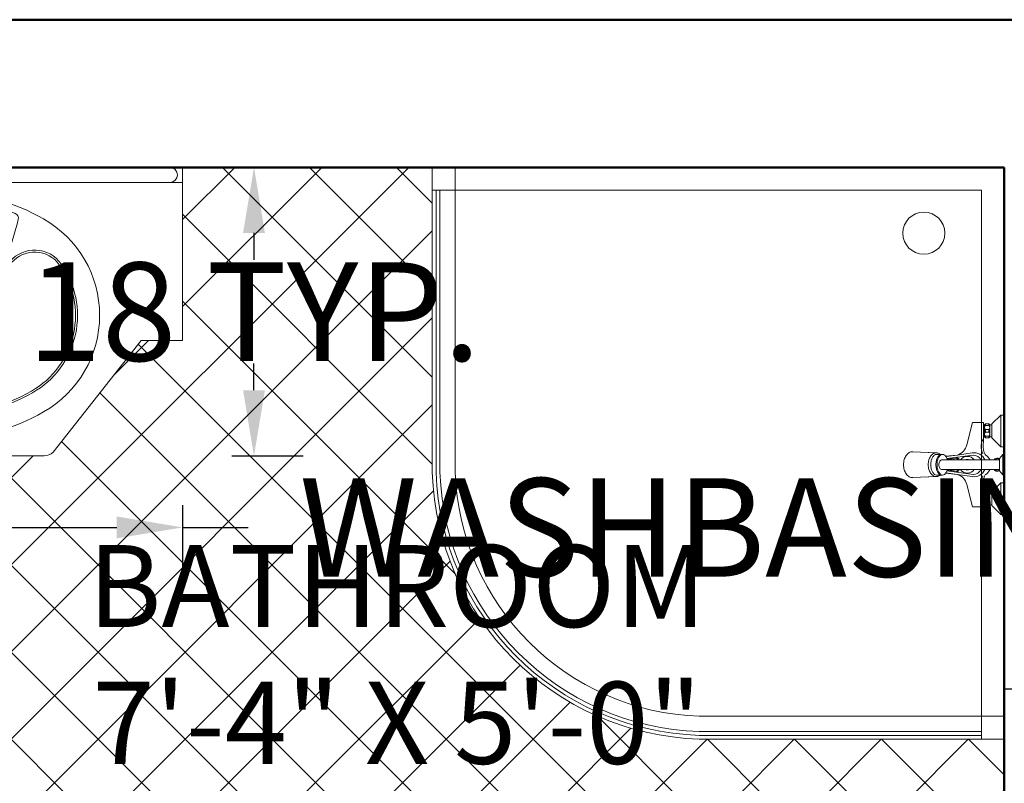
# Model space of a CAD drawing. Units: inches. Extents: x -466983 to 1020, y 324 to 318697.
# Tile 47 of 97: x 549 to 609, y 1038 to 1085. Entities that reach past the tile are written whole.
import ezdxf

# ---------------------------------------------------------------- set-up
doc = ezdxf.new("R2010")
doc.units = ezdxf.units.IN
doc.header["$MEASUREMENT"] = 0
for name, color, linetype, lineweight in [('A-ANNO-DIMS', 2, 'Continuous', 18), ('A-AREA-IDEN', 7, 'Continuous', 25), ('A-DOOR', 3, 'Continuous', 25), ('A-FLOR-FIXT', 9, 'Continuous', 18), ('A-FLOR-PATT', 252, 'Continuous', 13), ('A-GLAZ', 4, 'Continuous', 25), ('A-WALL', 7, 'Continuous', 50)]:
    doc.layers.add(name, color=color, linetype=linetype, lineweight=lineweight)
doc.styles.get("Standard").update_dxf_attribs({"font": 'arial.ttf'})
doc.dimstyles.get("Standard").update_dxf_attribs({"dimtxt": 6, "dimasz": 4, "dimexe": 3, "dimexo": 3, "dimgap": 0.09, "dimtad": 0, "dimtih": 1, "dimtoh": 1, "dimdec": 1, "dimzin": 0, "dimdsep": 46, "dimlunit": 3, "dimtxsty": 'Standard', "dimcen": 0.09, "dimadec": 0, "dimazin": 0, "dimtfac": 1, "dimtdec": 1, "dimtofl": 0, "dimtmove": 0, "dimatfit": 3, "dimfxl": 1, "dimtolj": 1, "dimtzin": 0, "dimarcsym": 0})

# ---------------------------------------------------------------- blocks, each defined once
blk = doc.blocks.new('Ventilator')
for p, q in [((1433.5927409432, 801.6799676286266), (1457.592740943201, 801.6799676286266)), ((1433.5927409432, 792.6799676286266), (1433.5927409432, 801.6799676286266)), ((1457.592740943201, 801.6799676286266), (1457.592740943201, 792.6799676286266)), ((1433.5927409432, 797.9799676286265), (1457.592740943201, 797.9799676286265)), ((1457.592740943201, 796.3799676286266), (1433.5927409432, 796.3799676286266)), ((1457.592740943201, 792.6799676286266), (1433.5927409432, 792.6799676286266))]:
    blk.add_line(p, q)
blk = doc.blocks.new('B1')
for p, q in [((0, 1300.000000000277), (693.3333333334303, 1300.000000000277)), ((0, 1.023182e-10), (0, 1300.000000000277)), ((52.00000000000727, 52.00000000000045), (52.00000000000727, 1300.000000000277)), ((52.00000000000727, 1291.33333333362), (693.3333333334303, 1291.33333333362)), ((52.00000000000727, 1282.666666666948), (693.3333333334303, 1282.666666666948)), ((0, 1248.000000000277), (693.3333333334303, 1248.000000000277)), ((140.3876720592416, 699.4289321882679), (154.4144116848583, 699.4289321882679)), ((208.8876720592416, 705.4289321882679), (153.4804125083301, 702.8756022550479)), ((21.99999999999818, 689.0000000001346), (21.99999999999818, 687.0000000001382)), ((1248.000000000174, 693.6609680139231), (1248.000000000174, 1.023182e-10)), ((1282.666666666846, 693.6609680139231), (1282.666666666846, 52.00000000010231)), ((1291.333333333514, 693.6609680139231), (1291.333333333517, 52.00000000010231)), ((1300.000000000182, 693.6609680139231), (1300.000000000182, 1.023182e-10)), ((21.99999999999818, 663.0000000001382), (21.99999999999818, 665.0000000001309)), ((140.3876720592416, 652.5710678120049), (154.4144116848583, 652.5710678120049)), ((208.8876720592416, 646.5710678120049), (153.5459520445456, 648.976381547378)), ((52.00000000001091, 52.00000000000045), (1300.000000000178, 52.00000000010231)), ((0, 4.547e-13), (1300.000000000182, 1.023182e-10))]:
    blk.add_line(p, q)
for points in [[(0, 775.000000000131), (0, 789.0000000001346), (8, 789.0000000001346)], [(8, 789.0000000001346), (8, 717.0000000001309)], [(8, 789.0000000001346), (27.99999999999818, 769.0000000001309), (27.99999999999818, 767.0000000001382)], [(0, 754.0000000001382), (0, 775.000000000131)], [(27.99999999999818, 767.0000000001382), (33.00000000000182, 767.0000000001382)], [(27.99999999999818, 767.0000000001382), (27.99999999999818, 753.0000000001345)], [(33.00000000000182, 767.0000000001382), (35, 769.0000000001309), (43, 769.0000000001309), (45.00000000000182, 767.0000000001382)], [(33.00000000000182, 767.0000000001382), (33.00000000000182, 753.0000000001345)], [(35, 765.0000000001345), (33.00000000000182, 762.0000000001346)], [(43, 769.0000000001309), (43, 765.0000000001345), (35, 765.0000000001345), (35, 769.0000000001309)], [(43, 765.0000000001345), (45.00000000000182, 763.0000000001382)], [(47, 767.0000000001382), (45.00000000000182, 767.0000000001382)], [(45.00000000000182, 767.0000000001382), (45.00000000000182, 753.0000000001345)], [(47, 739.0000000001382), (47, 767.0000000001382)], [(8, 717.0000000001309), (0, 717.0000000001309), (0, 754.0000000001382)], [(8, 717.0000000001309), (27.99999999999818, 737.0000000001346), (27.99999999999818, 739.0000000001382)], [(27.99999999999818, 739.0000000001382), (27.99999999999818, 753.0000000001345)], [(27.99999999999818, 739.0000000001382), (33.00000000000182, 739.0000000001382)], [(33.00000000000182, 758.0000000001346), (35, 756.0000000001346), (43, 756.0000000001346), (45.00000000000182, 758.0000000001346)], [(33.00000000000182, 739.0000000001382), (33.00000000000182, 753.0000000001345)], [(33.00000000000182, 748.0000000001382), (35, 750.0000000001346), (43, 750.0000000001346), (45.00000000000182, 748.0000000001382)], [(35, 741.0000000001346), (33.00000000000182, 744.0000000001345)], [(33.00000000000182, 739.0000000001382), (35, 737.0000000001346), (43, 737.0000000001346), (45.00000000000182, 739.0000000001382)], [(35, 756.0000000001346), (35, 753.0000000001345)], [(35, 750.0000000001346), (35, 753.0000000001345)], [(43, 737.0000000001346), (43, 741.0000000001346), (35, 741.0000000001346), (35, 737.0000000001346)], [(43, 756.0000000001346), (43, 753.0000000001345)], [(43, 750.0000000001346), (43, 753.0000000001345)], [(43, 741.0000000001346), (45.00000000000182, 743.0000000001346)], [(45.00000000000182, 739.0000000001382), (45.00000000000182, 753.0000000001345)], [(47, 739.0000000001382), (45.00000000000182, 739.0000000001382)], [(47, 728.0000000001345), (47, 739.0000000001382)], [(0, 687.0000000001382), (0, 699.0000000001382)], [(0, 699.0000000001382), (3, 699.0000000001382)], [(3, 699.0000000001382), (3, 676.0000000001346)], [(3, 699.0000000001382), (11, 690.0000000001382), (11, 687.0000000001382)], [(0, 665.0000000001309), (0, 687.0000000001382)], [(3, 653.0000000001309), (3, 676.0000000001346)], [(11, 687.0000000001382), (11, 676.0000000001346)], [(140.9999999999982, 687.0000000001382), (11, 687.0000000001382)], [(11, 665.0000000001309), (11, 676.0000000001346)], [(0, 653.0000000001309), (0, 665.0000000001309)], [(0, 653.0000000001309), (3, 653.0000000001309)], [(3, 653.0000000001309), (11, 662.000000000131), (11, 665.0000000001309)], [(140.9999999999982, 665.0000000001309), (11, 665.0000000001309)], [(133.9221670278657, 656.0563042479444), (133.0620831697051, 656.0563042479444)], [(7.999999999998181, 635.0000000001382), (0, 635.0000000001382), (0, 598.0000000001309)], [(7.999999999998181, 563.0000000001346), (7.999999999998181, 635.0000000001382)], [(7.999999999998181, 635.0000000001382), (27.99999999999818, 615.0000000001345), (27.99999999999818, 613.0000000001346)], [(27.99999999999818, 613.0000000001346), (27.99999999999818, 599.0000000001382)], [(27.99999999999818, 613.0000000001346), (33.00000000000182, 613.0000000001346)], [(33.00000000000182, 613.0000000001346), (35, 615.0000000001345), (42.99999999999818, 615.0000000001345), (45.00000000000182, 613.0000000001346)], [(33.00000000000182, 613.0000000001346), (33.00000000000182, 599.0000000001382)], [(35, 611.0000000001382), (33.00000000000182, 608.0000000001382)], [(42.99999999999818, 615.0000000001345), (42.99999999999818, 611.0000000001382), (35, 611.0000000001382), (35, 615.0000000001345)], [(42.99999999999818, 611.0000000001382), (45.00000000000182, 609.0000000001346)], [(45.00000000000182, 613.0000000001346), (45.00000000000182, 599.0000000001382)], [(47, 613.0000000001346), (45.00000000000182, 613.0000000001346)], [(47, 624.0000000001345), (47, 613.0000000001346)], [(47, 613.0000000001346), (47, 585.0000000001346)], [(0, 598.0000000001309), (0, 577.0000000001382)], [(7.999999999998181, 563.0000000001346), (27.99999999999818, 583.000000000131), (27.99999999999818, 585.0000000001346)], [(27.99999999999818, 585.0000000001346), (27.99999999999818, 599.0000000001382)], [(27.99999999999818, 585.0000000001346), (33.00000000000182, 585.0000000001346)], [(33.00000000000182, 604.0000000001346), (35, 602.0000000001382), (42.99999999999818, 602.0000000001382), (45.00000000000182, 604.0000000001346)], [(33.00000000000182, 585.0000000001346), (33.00000000000182, 599.0000000001382)], [(33.00000000000182, 594.0000000001345), (35, 596.0000000001382), (42.99999999999818, 596.0000000001382), (45.00000000000182, 594.0000000001345)], [(35, 587.0000000001382), (33.00000000000182, 590.0000000001382)], [(33.00000000000182, 585.0000000001346), (35, 583.000000000131), (42.99999999999818, 583.000000000131), (45.00000000000182, 585.0000000001346)], [(35, 602.0000000001382), (35, 599.0000000001382)], [(35, 596.0000000001382), (35, 599.0000000001382)], [(42.99999999999818, 583.000000000131), (42.99999999999818, 587.0000000001382), (35, 587.0000000001382), (35, 583.000000000131)], [(42.99999999999818, 602.0000000001382), (42.99999999999818, 599.0000000001382)], [(42.99999999999818, 596.0000000001382), (42.99999999999818, 599.0000000001382)], [(42.99999999999818, 587.0000000001382), (45.00000000000182, 589.0000000001309)], [(45.00000000000182, 585.0000000001346), (45.00000000000182, 599.0000000001382)], [(47, 585.0000000001346), (45.00000000000182, 585.0000000001346)], [(0, 577.0000000001382), (0, 563.0000000001346), (7.999999999998181, 563.0000000001346)]]:
    blk.add_lwpolyline(points)
blk.add_lwpolyline([(208.8876720592416, 646.5710678120049), (154.6376720593016, 648.9289321882679, -0.1383183006310921), (148.063043746286, 650.7831906028294, -0.0370381408635636), (145.578855038857, 652.5710678120049), (140.3876720592379, 652.5710678120049, -0.1665558057867227), (136.092755137337, 654.0425753596318, -0.0535717192020755), (133.4948936773198, 656.547585930646), (107, 654.0000000001382, 0.2625940722123521), (85, 631.0000000001346), (72, 580.0000000001419), (47, 580.0000000001419), (47, 585.0000000001346), (45.00000000000182, 585.0000000001346), (42.99999999999818, 583.0000000001346), (35, 583.0000000001346), (33.00000000000182, 585.0000000001346), (27.99999999999818, 585.0000000001346), (27.99999999999818, 583.0000000001346), (7.999999999998181, 563.0000000001382), (0, 563.0000000001382), (0, 577.0000000001418), (0, 598.0000000001346), (0, 635.0000000001418), (7.999999999998181, 635.0000000001418), (27.99999999999818, 615.0000000001382), (27.99999999999818, 613.0000000001346), (33.00000000000182, 613.0000000001346), (35, 615.0000000001382), (42.99999999999818, 615.0000000001382), (45.00000000000182, 613.0000000001346), (47, 613.0000000001346), (47, 624.0000000001382, 0.1247866838288863), (46, 648.0000000001382, 0.1501483781683498), (42.00000000000182, 654.0000000001382, -0.1384844099870248), (32.50754085593508, 665.0000000001345), (21.99999999999818, 665.0000000001345), (21.99999999999818, 663.0000000001382, -0.3003468456066685), (11, 662.3397459768711), (11, 662.0000000001346), (3, 653.0000000001345), (0, 653.0000000001345), (0, 665.0000000001345), (0, 687.0000000001382), (0, 699.0000000001418), (3, 699.0000000001418), (11, 690.0000000001382), (10.99999999999636, 689.6602540496569, -0.3003468456580443), (21.99999999999818, 689.0000000001346), (21.99999999999818, 687.0000000001382), (32.50754085593508, 687.0000000001382, -0.138484409987018), (42.00000000000182, 698.0000000001346, 0.1501483781683498), (46, 704.0000000001346, 0.1247866838288863), (47, 728.0000000001382), (47, 739.0000000001382), (45.00000000000182, 739.0000000001382), (43, 737.0000000001382), (35, 737.0000000001382), (33.00000000000182, 739.0000000001382), (27.99999999999818, 739.0000000001382), (27.99999999999818, 737.0000000001382), (8, 717.0000000001346), (0, 717.0000000001346), (0, 754.0000000001382), (0, 775.0000000001346), (0, 789.0000000001382), (8, 789.0000000001382), (27.99999999999818, 769.0000000001345), (27.99999999999818, 767.0000000001382), (33.00000000000182, 767.0000000001382), (35, 769.0000000001345), (43, 769.0000000001345), (45.00000000000182, 767.0000000001382), (47, 767.0000000001382), (47, 772.0000000001346), (72, 772.0000000001346), (85, 721.0000000001382, 0.2625940722123521), (107, 698.0000000001346), (133.494893670435, 695.4524140702815, -0.0535717192022979), (136.092755137337, 697.9574246406409, -0.1665558057868109), (140.3876720592416, 699.4289321882679), (145.7502000114491, 699.4289321882679, -0.0343443404771406), (148.063043746286, 701.07467377371, -0.1383183006298331), (154.6376720592416, 702.9289321882715), (208.8876720591488, 705.4289321882679, -0.1377032461334603), (216.0999264221609, 703.4042378869926, -0.1070360850488126), (223.0298076829695, 696.809397513447, -0.0808015121757586), (227.273223711496, 687.6931912444343, -0.0687078013104136), (228.8876720592398, 676.0000000001382, -0.0687078013104135), (227.273223711496, 664.3068087558385, -0.0808015121757595), (223.0298076829695, 655.1906024868258, -0.107036085048811), (216.0999264221609, 648.5957621132802, -0.1377032461317454)], format="xyb", close=True)
for points in [[(47, 767.0000000001382), (47, 772.0000000001309), (72, 772.0000000001309), (85, 721.0000000001382, 0.2625940722123521), (107, 698.0000000001346), (133.4948936704422, 695.4524140702887, -0.3591123035969264)], [(47, 728.0000000001345, -0.1247866838288863), (46, 704.0000000001346, -0.1501483781683498), (42.00000000000182, 698.0000000001346, 0.138484409987018), (32.50754085593508, 687.0000000001382, 0.7633705308853952)], [(47, 734.0000000001346, -0.2052577019546359), (52, 726.0000000001309, -0.1374236490949136), (49, 701.0000000001346, -5.029096516974528)], [(106.0000000000018, 698.0000000001346), (73, 703.0000000001382, 0.3410628393219512), (44.19402075297876, 687.0000000001382, 0.987420997957196)], [(71.00000000000182, 698.0000000001346, 0.2653451188970793), (52.73167562087656, 687.0000000001382, 0.6855978624637613)], [(71.00000000000182, 698.0000000001346), (130.3767751999166, 690.0830966401517, -0.389881551935721)], [(106.0000000000018, 698.0000000001346), (132.9051195245556, 694.7054955685562, -0.3445125279727503)], [(129.2869436463206, 665.0799945585786, 0.0546118951167688), (131.5488372944073, 659.4332431739494, 0.1055200220071626), (136.092755137337, 654.0425753596318, 0.1665558057868128), (140.3876720592416, 652.5710678120049, 0.1665558057868108), (144.6825889811407, 654.0425753596318, 0.1055200220071628), (149.2265068240704, 659.4332431739494, 0.0682582856346859), (151.8562849435693, 666.5533485092964, 0.0544283700167335), (152.8876720592398, 676.0000000001346, 0.0544283700167333), (151.8562849435693, 685.4466514909764, 0.0682582856346864), (149.2265068240704, 692.5667568263307, 0.1055200220071624), (144.6825889811407, 697.9574246406409, 0.1665558057868127), (140.3876720592416, 699.4289321882679, 0.1665558057868109), (136.092755137337, 697.9574246406409, 0.1055200220071607), (131.5488372944073, 692.5667568263307, 0.0538660454735237), (129.3093729212014, 687.0000000001382, 0.0544283700167342)], [(141.6455361051521, 652.6849517968694, 0.0451764077839428), (142.9034001510663, 652.5710678120049, 0.1665558057868108), (147.1983170729654, 654.0425753596318, 0.1055200220071628), (151.7422349158969, 659.4332431739494, 0.0682582856346859), (154.3720130353958, 666.5533485092964, 0.0544283700167335), (155.4034001510663, 676.0000000001346, 0.0544283700167333), (154.3720130353958, 685.4466514909764, 0.0682582856346864), (151.7422349158969, 692.5667568263307, 0.1055200220071624), (147.1983170729654, 697.9574246406409, 0.1665558057868127), (142.9034001510663, 699.4289321882679, 0.0451764077839423), (141.6455361051521, 699.315048203407, 0.1055200220071607)], [(145.5788550388533, 652.5710678120049, 0.0370381408635636), (148.063043746286, 650.7831906028294, 0.1383183006298338), (154.6376720592416, 648.9289321882679, 0.138318300629834), (161.2123003721917, 650.7831906028294, 0.1070627939593127), (167.5423708158942, 656.8370490962297, 0.0805227312927088), (171.4136097265637, 665.1966168081926, 0.0683531574638633), (172.8876720592398, 675.9289321882679, 0.0683531574638646), (171.4136097265637, 686.6612475683432, 0.0805227312927094), (167.5423708158942, 695.0208152803061, 0.1070627939593105), (161.2123003721917, 701.07467377371, 0.1383183006298341), (154.6376720592416, 702.9289321882715, 0.1383183006298331), (148.063043746286, 701.07467377371, 0.0343443404771406), (145.7502000114491, 699.4289321882679, 0.0805227312927093)], [(154.4144116848583, 652.5710678120049, 0.1665558057868108), (158.7093286067611, 654.0425753596318, 0.1055200220071628), (163.2532464496908, 659.4332431739494, 0.0682582856346859), (165.8830245691897, 666.5533485092964, 0.0544283700167335), (166.9144116848601, 676.0000000001346, 0.0544283700167333), (165.8830245691897, 685.4466514909764, 0.0682582856346864), (163.2532464496908, 692.5667568263307, 0.1055200220071624), (158.7093286067611, 697.9574246406409, 0.1665558057868127), (154.4144116848583, 699.4289321882679, 0.1665558057868109)], [(207.6853336958775, 646.6233249695179, 0.0217212157548433), (208.8876720592416, 646.5710678120049, 0.1377032461317454), (216.0999264221609, 648.5957621132802, 0.107036085048811), (223.0298076829695, 655.1906024868258, 0.0808015121757595), (227.273223711496, 664.3068087558385, 0.0687078013104135), (228.8876720592398, 676.0000000001346, 0.0687078013104136), (227.273223711496, 687.6931912444343, 0.0808015121757586), (223.0298076829695, 696.809397513447, 0.1070360850488126), (216.0999264221609, 703.4042378869926, 0.1377032461317515), (208.8876720592416, 705.4289321882679, 0.0115815460008583), (208.2459469633304, 705.4140658567775, 0.1070360850488107)], [(11, 688.0000000001346, -0.2034527507076884), (11.27314869702968, 688.6434964536201, -0.0971632324952149), (12.46446609406666, 689.4142135625043, -0.0541309211895364), (13.96123847455419, 689.8322469457524, -0.041071521782227), (15.99999999999818, 690.0000000001382, -0.041071521782232), (18.03876152544581, 689.8322469457524, -0.0541309211895581), (19.53553390593333, 689.4142135625043, -0.0971632324952149), (20.72685130297032, 688.6434964536201, -0.2034527507076884), (21, 688.0000000001346, -0.2034527507076693), (20.72685130297032, 687.3565035466526, -0.0379533313060429), (20.29672106629732, 687.0000000001382, -0.0541309211895384)], [(11.70327893370086, 687.0000000001382, -0.0379533313059558), (11.27314869702968, 687.3565035466526, -0.2034527507076722), (11, 688.0000000001346, -0.2034527507076884)], [(11.14357068821118, 689.7415727613479, -0.2958552022276962), (21.99999999999818, 689.0000000001346, -2.290285352134018)], [(109.0000000000018, 693.0000000001382, 0.3394066855219726), (103.0542662941007, 687.0000000001382)], [(105.3371881863113, 687.0000000001382, -0.2701562118716146), (110, 691.0000000001346), (129.6983785438242, 688.2641140912746, -0.3982822486971544)], [(140.9999999999982, 665.0000000001309, 0.130158640187584), (143.919967274478, 665.7732172227988, 0.1064685849763611), (146.6568542494933, 668.2218254070867, 0.0842476149744631), (148.3593095850538, 671.6519929664936, 0.0732806852421333), (149, 676.0000000001346, 0.0732806852421325), (148.3593095850538, 680.3480070337755, 0.0842476149744645), (146.6568542494933, 683.7781745931861, 0.1064685849763632), (143.919967274478, 686.226782777474, 0.1301586401875921), (140.9999999999982, 687.0000000001382, 0.1301586401875932)], [(11, 664.0000000001346, 0.2034527507076884), (11.27314869702968, 663.356503546649, 0.0971632324952149), (12.46446609406666, 662.5857864377649, 0.0541309211895364), (13.96123847455419, 662.1677530545167, 0.041071521782227), (15.99999999999818, 662.000000000131, 0.041071521782232), (18.03876152544581, 662.1677530545167, 0.0541309211895581), (19.53553390593333, 662.5857864377649, 0.0971632324952149), (20.72685130297032, 663.356503546649, 0.2034527507076884), (21, 664.0000000001346, 0.2034527507076693), (20.72685130297032, 664.6434964536202, 0.0379533313062782), (20.29672106629369, 665.0000000001309, 0.0541309211895384)], [(11.70327893370449, 665.0000000001309, 0.0379533313061481), (11.27314869702968, 664.6434964536202, 0.2034527507076722), (11, 664.0000000001346, 0.2034527507076884)], [(11.14357068821118, 662.2584272389249, 0.2958552022276962), (21.99999999999818, 663.0000000001382, 2.290285352134018)], [(47, 624.0000000001345, 0.1247866838288863), (46, 648.0000000001382, 0.1501483781683498), (42.00000000000182, 654.0000000001382, -0.1384844099870248), (32.50754085593508, 665.0000000001309, -0.7633705308853952)], [(106.0000000000018, 654.0000000001382), (73, 649.0000000001345, -0.341062839321959), (44.19402075297876, 665.0000000001309, -0.987420997957196)], [(47, 585.0000000001346), (47, 580.0000000001382), (72, 580.0000000001382), (85, 631.0000000001346, -0.2625940722123521), (107, 654.0000000001382), (132.4235230446356, 656.4445695236572, 0.3591123035969264)], [(47, 618.0000000001346, 0.2052577019546359), (52, 626.0000000001382, 0.1374236490949136), (49, 651.0000000001382, 5.029096516974528)], [(71.00000000000182, 654.0000000001382, -0.2653451188970914), (52.73167562087656, 665.0000000001309, -0.6855978624637613)], [(71.00000000000182, 654.0000000001382), (130.3767751999166, 661.9169033601211, 0.389881551935721)], [(109.0000000000018, 659.0000000001309, -0.3394066855220244), (103.0542662941007, 665.0000000001309)], [(105.3371881863113, 665.0000000001309, 0.2701562118716416), (110, 661.0000000001345), (129.6983785438278, 663.7358859089982, 0.3982822486971544)], [(106.0000000000018, 654.0000000001382), (132.9051195245556, 657.2945044317166, 0.3445125279727503)]]:
    blk.add_lwpolyline(points, format="xyb")
blk.add_circle((182.931355266388, 149.5974501754249), 47.86997641275996)
for centre, radius, start, end in [((672.5535632588981, 672.5422464127919), 627.8017452838134, 1.92774542086775, 88.10320593202876), ((672.5535632588981, 672.5422464127919), 610.4684119504776, 1.92774542086775, 88.10320593202876), ((672.5535632588981, 672.5422464127919), 619.1350786171454, 1.92774542086775, 88.10320593202876), ((672.5535632588981, 672.5422464127919), 575.801745283806, 1.92774542086775, 88.10320593202876), ((84, 676.0000000001346), 19, 35.37654015188604, 144.6234598481139), ((84, 676.0000000001346), 12.00000000000001, 66.44353569094163, 113.5564643090584), ((120.8125, 676.1250000001309), 12.8131097415889, 112.0608994672246, 121.9251013585072), ((123.9999999999982, 676.0000000001346), 13, 64.79528984039216, 122.2042275039623), ((84, 676.0000000001346), 19, 215.376540151886, 324.623459848114), ((84, 676.0000000001346), 12.00000000000001, 246.4435356909416, 293.5564643090584), ((120.8125, 675.8750000001382), 12.8131097415889, 238.0748986414927, 247.9391005327754), ((123.9999999999982, 676.0000000001346), 13, 237.7957724960376, 295.2047101596079)]:
    blk.add_arc(centre, radius, start, end)
blk = doc.blocks.new('*U38')
for p, q in [((0, 0), (-1.1e-15, 5.999999999999999)), ((40, 8e-15), (40, 6.000000000000007))]:
    blk.add_line(p, q)
blk.add_lwpolyline([(0, 0), (1.42e-14, -40), (1.750000000000014, -40), (1.75, 9e-16)], close=True)
blk.add_arc((0, 0), 40, 270, 0)
blk = doc.blocks.new('B3')
for p, q in [((-450, 0), (-455.7402514854766, -1.1418070123309)), ((450, 0), (455.7402514854766, -1.1418070123309)), ((-463.8581929876745, -9.25974851452338), (-465, -15)), ((-465, -15), (-463.8581929876745, -20.74025148547662)), ((-460.6066017178018, -4.393398282201815), (-463.8581929876745, -9.25974851452338)), ((-455.7402514854766, -1.1418070123309), (-460.6066017178018, -4.393398282201815)), ((455.7402514854766, -1.1418070123309), (460.6066017177945, -4.393398282201815)), ((460.6066017177945, -4.393398282201815), (463.8581929876672, -9.25974851452338)), ((463.8581929876672, -9.25974851452338), (465, -15)), ((465, -15), (463.8581929876672, -20.74025148547662)), ((475, -30), (-475, -30)), ((-463.8581929876745, -20.74025148547662), (-460.6066017178018, -25.60660171779819)), ((-460.6066017178018, -25.60660171779819), (-455.7402514854766, -28.8581929876691)), ((-455.7402514854766, -28.8581929876691), (-450, -30)), ((455.7402514854766, -28.8581929876691), (450, -30)), ((460.6066017177945, -25.60660171779819), (455.7402514854766, -28.8581929876691)), ((463.8581929876672, -20.74025148547662), (460.6066017177945, -25.60660171779819)), ((2.91038e-11, -182.0000000000054), (-115.8117069986983, -182.0000000000054)), ((2.91038e-11, -182.0000000000054), (115.8117069987565, -182.0000000000054))]:
    blk.add_line(p, q)
blk.add_lwpolyline([(199.4833683843535, -575, 0.2017697719241106), (217.3542190239823, -567.482353886593), (392.5, -345), (435, -345), (475, -345), (475, 0), (-475, 0), (-475, -345), (-435, -345), (-392.5, -345), (-217.3542190239896, -567.482353886593, 0.2017697719241107), (-199.4833683843608, -575)], format="xyb", close=True)
for centre, radius, start, end in [((5.09317e-11, -450.0000000000327), 400.0000000000322, 90, 119.7172288959075), ((0, -450.0000000000327), 400.0000000000319, 60.28277110409252, 90), ((2.91038e-11, -450.0000000000055), 385, 90, 111.6513567404431), ((2.91038e-11, -450.0000000000055), 385, 68.34864325955687, 90), ((-138.3591766736499, -101.4576952073475), 10, 111.6513567404431, 193.3915177581575), ((138.3591766737008, -101.4576952073475), 10, 346.6084822418425, 68.34864325955687), ((-88.47222222221171, -295.0000000000055), 221.527777777762, 119.7172288959075, 240.2827711040925), ((338.3178096717893, 12.0282100348104), 500, 193.3915177581575, 202.0594091764406), ((-338.3178096717383, 12.0282100348104), 500, 337.9405908235594, 346.6084822418425), ((88.47222222225537, -294.9999999999964), 221.527777777762, 299.7172288959074, 60.28277110409252), ((2.91038e-11, -136.9999999999891), 17.5, 90, 270), ((2.91038e-11, -136.9999999999891), 17.5, 270, 90), ((-180.5137974189128, -229.2550553338115), 64.41699441097052, 40.71477974361456, 144.4619255202982), ((-180.5137974189128, -229.2550553338115), 60.41699441097051, 40.71477974361456, 144.4619255202982), ((-115.8117069986983, -172.0000000000145), 10, 202.0594091764406, 270), ((115.8117069987565, -172.0000000000145), 10, 270, 337.9405908235594), ((180.5137974189638, -229.2550553338115), 64.41699441097052, 35.53807447970174, 139.2852202563854), ((180.5137974189638, -229.2550553338115), 60.41699441097051, 35.53807447970174, 139.2852202563854), ((-88.47222222221171, -295.0000000000055), 177.5277777777778, 144.4619255202982, 240.2827711040925), ((-88.47222222221171, -295.0000000000055), 173.5277777777778, 144.4619255202982, 240.2827711040925), ((88.47222222223354, -295.0000000000055), 173.5277777777778, 299.7172288959074, 35.53807447970174), ((88.47222222223354, -295.0000000000055), 177.5277777777778, 299.7172288959074, 35.53807447970174), ((2.91038e-11, -247.0000000000037), 37.5, 90, 270), ((2.91038e-11, -247.0000000000037), 37.5, 270, 90), ((2.91038e-11, -247.0000000000037), 23, 90, 270), ((2.91038e-11, -247.0000000000037), 23, 270, 90), ((2.91038e-11, -140.0000000000036), 356, 240.2827711040925, 270), ((2.91038e-11, -140.0000000000036), 352, 240.2827711040925, 270), ((2.91038e-11, -140.0000000000036), 352, 270, 299.7172288959074), ((2.91038e-11, -140.0000000000036), 356, 270, 299.7172288959074), ((5.09317e-11, -139.9999999999781), 400.0000000000309, 240.2827711040925, 270), ((-1.45519e-11, -140.0000000000309), 399.9999999999781, 270, 299.7172288959074)]:
    blk.add_arc(centre, radius, start, end)
blk = doc.blocks.new('*D79')
at = {"layer": 'A-ANNO-DIMS', "color": 0, "lineweight": -2, "transparency": 16777216}
for p, q in [((529.6742726119846, 1055.350891982691), (529.6742726119846, 1050.992414036445)), ((558.7307922536265, 1055.350891982691), (558.7307922536265, 1050.992414036445)), ((533.6742726119846, 1053.992414036445), (554.7307922536265, 1053.992414036445)), ((558.7307922536265, 1053.992414036445), (562.7307922536265, 1053.992414036445))]:
    blk.add_line(p, q, dxfattribs=at)
at = {"layer": 'A-ANNO-DIMS', "color": 0, "transparency": 16777216}
for points in [[(533.6742726119846, 1054.659080703112), (533.6742726119846, 1053.325747369778), (529.6742726119846, 1053.992414036445)], [(554.7307922536265, 1054.659080703112), (554.7307922536265, 1053.325747369778), (558.7307922536265, 1053.992414036445)]]:
    blk.add_solid(points, dxfattribs=at)
at = {"layer": 'Defpoints', "color": 0, "transparency": 16777216}
for p in [(529.6742726119846, 1058.350891982691), (558.7307922536265, 1058.350891982691), (558.7307922536265, 1053.992414036445)]:
    blk.add_point(p, dxfattribs=at)
at = {"layer": 'A-ANNO-DIMS', "color": 0, "transparency": 16777216, "insert": (603.861037819793, 1053.992414036445), "char_height": 6, "attachment_point": 5}
blk.add_mtext('\\A1;WASHBASIN 29 TYP.', dxfattribs=at)
blk = doc.blocks.new('*D80')
at = {"layer": 'A-ANNO-DIMS', "color": 0, "lineweight": -2, "transparency": 16777216}
for p, q in [((561.7307922536268, 1075.937732818422), (566.0892701998732, 1075.937732818422)), ((563.0892701998732, 1071.937732818422), (563.0892701998732, 1070.297750326887)), ((563.0892701998732, 1062.350891982692), (563.0892701998732, 1063.990874474227)), ((561.7307922536268, 1058.350891982692), (566.0892701998732, 1058.350891982692))]:
    blk.add_line(p, q, dxfattribs=at)
at = {"layer": 'A-ANNO-DIMS', "color": 0, "transparency": 16777216}
for points in [[(562.4226035332066, 1071.937732818422), (563.7559368665399, 1071.937732818422), (563.0892701998732, 1075.937732818422)], [(562.4226035332066, 1062.350891982692), (563.7559368665399, 1062.350891982692), (563.0892701998732, 1058.350891982692)]]:
    blk.add_solid(points, dxfattribs=at)
at = {"layer": 'Defpoints', "color": 0, "transparency": 16777216}
for p in [(558.7307922536266, 1075.937732818422), (563.0892701998732, 1075.937732818422), (558.7307922536266, 1058.350891982692)]:
    blk.add_point(p, dxfattribs=at)
at = {"layer": 'A-ANNO-DIMS', "color": 0, "transparency": 16777216, "insert": (563.0892701998735, 1067.144312400557), "char_height": 6, "attachment_point": 5}
blk.add_mtext('\\A1;18 TYP.', dxfattribs=at)

msp = doc.modelspace()

# ---------------------------------------------------------------- hatches: boundary and pattern name
at = {"layer": 'A-FLOR-PATT', "transparency": 33554572}
h = msp.add_hatch(dxfattribs=at)
h.set_pattern_fill('ANSI37', color=256, scale=30)
h.set_pattern_definition([(45, (-1212.413693079869, -290.0350025265127), (-2.651650429449553, 2.651650429449553), []), (135, (-1212.413693079869, -290.0350025265127), (-2.651650429449553, -2.651650429449552), [])])
h.paths.add_polyline_path([(901.805677520904, 1075.937732818422), (900.6144036774049, 1075.937732818422), (900.6144036774049, 1065.385628316983), (899.390971271441, 1065.385628316983), (898.0910743401043, 1065.385628316983), (892.8355944880973, 1058.709752245277, -0.2583770168556315), (892.18750428989, 1058.350891982691), (879.9847834232776, 1058.350891982691, -0.2017697719240963), (879.438188978411, 1058.580825279484), (874.0812133730635, 1065.385628316983), (872.7813164417267, 1065.385628316983), (871.5578840357629, 1065.385628316983), (871.5578840357629, 1075.937732818422), (813.8056775209042, 1075.937732818422), (813.8056775209042, 1044.792233318721), (832.3947444543938, 1044.792233318721, -0.3947951267487684), (848.6601780212009, 1028.535584015862), (848.6601780212009, 1009.937732818421), (901.805677520904, 1009.937732818421), (901.805677520904, 1015.937732818421), (901.3056775209042, 1015.937732818421), (871.3056775209039, 1015.937732818421), (871.3056775209039, 1017.250232818421), (871.3344022102003, 1017.250232818421, -0.4014527144963572), (901.3056775209042, 1045.937732818421), (901.805677520904, 1045.937732818421)])
edge = h.paths.add_edge_path(flags=16)
edge.add_line((847.7730719745084, 1068.948588737025), (847.7730719745069, 1073.708823774771))
edge.add_arc((849.2268986539951, 1073.708823774771), 1.453826679487974, 90, 180, ccw=False)
edge.add_line((849.2268986539951, 1075.162650454259), (864.4920787886183, 1075.162650454259))
edge.add_arc((864.4920787886213, 1073.708823774771), 1.453826679487974, 0, 90.00000000012102, ccw=False)
edge.add_line((865.9459054681093, 1073.708823774771), (865.9459054681081, 1069.00351244647))
edge.add_arc((832.6447385074767, 1068.976050591752), 33.30117828385809, -20.61233806670998, 0.04724903539101888, ccw=False)
edge.add_ellipse((856.8594887213083, 1058.479989307073), major_axis=(-2.091e-13, 10.21313242340307), ratio=0.6859192225533502, start_angle=100.00884331843292, end_angle=259.9911566815624, ccw=False)
edge.add_arc((881.0742389351396, 1068.976050591752), 33.30117828385809, 180.0472490354062, 200.6123380667097, ccw=False)
h.paths.add_polyline_path([(853.145578187156, 1066.481532374271), (853.145578187156, 1066.453444752512), (853.1463399851561, 1066.453444752512, 0.4331071439582673), (852.9166149812349, 1066.684892837266), (852.9166149812349, 1066.453444752512), (853.145578187156, 1066.453444752512), (853.145578187156, 1066.481532374489), (853.088019486549, 1066.612171966583, 0.6979386910037918), (852.699540939094, 1066.453444752512), (852.7003027371272, 1066.453444752512), (852.7003027371272, 1066.481532374489), (852.9166149812349, 1067.001204630995), (852.9166149812349, 1066.684892837266, -0.3962543063594317)], flags=0)
h.paths.add_polyline_path([(861.0186747055222, 1066.481532374271), (861.0186747055222, 1066.453444752512), (861.0194365035225, 1066.453444752512, 0.4164039232557909), (860.8023624614146, 1066.684892837265), (860.8023624614146, 1066.453444752512), (861.0186747055222, 1066.453444752512), (861.0186747055222, 1066.481532374489), (860.9671752720659, 1066.605255499379, 0.7133437187663149), (860.5726374574602, 1066.453444752512), (860.5733992554934, 1066.453444752512), (860.5733992554934, 1066.481532374489), (860.8023624614146, 1067.001204630995), (860.8023624614146, 1066.684892837265, -0.3799725304814568)], flags=0)
edge = h.paths.add_edge_path(flags=0)
edge.add_spline(control_points=[(861.1298377106021, 1065.785468371534), (861.4660965533383, 1065.247811229462), (861.613385559155, 1065.016139861057), (861.9832837951076, 1064.373617117607), (862.1924105327118, 1063.944313665492), (862.5613774174725, 1063.039129539609), (862.7212131906668, 1062.56326642291), (862.9865156700853, 1061.578122280975), (863.0919804897928, 1061.068856600952), (863.2452407883674, 1060.031049745086), (863.293035446714, 1059.502522766744), (863.3294736797056, 1058.440879580113), (863.3181170778639, 1057.907777155726), (863.2366033468288, 1056.85179603536), (863.1664466211855, 1056.328931215311), (862.9695120306455, 1055.307951977375), (862.8427353108815, 1054.809852090196), (862.5365466723708, 1053.852219447362), (862.3571373353129, 1053.392702749349), (861.9514237071658, 1052.524888245794), (861.7251255454219, 1052.116609101398), (861.2330086320977, 1051.362239687588), (860.9672044472572, 1051.016170456457), (860.4047960485765, 1050.394909316517), (860.1082220871676, 1050.119734477926), (859.493696255806, 1049.64606200509), (859.1757900615103, 1049.447558762665), (858.5275631429041, 1049.129883644436), (858.197273503909, 1049.010664382187), (857.5314773710529, 1048.851811036626), (857.1959384637446, 1048.812116564677), (856.5249326641573, 1048.811967422545), (856.1893892160524, 1048.851512676201), (855.5235728169741, 1049.010066967686), (855.1932673158994, 1049.129136347874), (854.5449932971788, 1049.446513839261), (854.2270557868354, 1049.644869411481), (853.6124495619564, 1050.118254324803), (853.3158265363004, 1050.393289340464), (852.7533025914207, 1051.014284587242), (852.487431959371, 1051.360227769297), (851.9951668313728, 1052.114363776776), (851.7687869247744, 1052.522535562859), (851.3628973914427, 1053.390157753425), (851.1833939042357, 1053.849589492002), (850.8770077813263, 1054.807077270704), (850.7501277313783, 1055.30511724975), (850.5529806633081, 1056.326003473117), (850.4827147921034, 1056.848835185142), (850.4009803807432, 1057.904777820697), (850.3895122452288, 1058.437874867502), (850.425728471152, 1059.499535178563), (850.4734126571939, 1060.02808465918), (850.6264565107679, 1061.065963770327), (850.7318153592672, 1061.575279204679), (850.9969137893603, 1062.560548677974), (851.1566514873134, 1063.036487374614), (851.525433403113, 1063.94184619004), (851.7344732542367, 1064.371248757046), (852.1056260411488, 1065.016350037675), (852.2544071072941, 1065.250281998093), (852.608154630964, 1065.733465727338)], knot_values=[3.915332106759953, 3.915332106759953, 3.915332106759953, 3.915332106759953, 4.013467662305501, 4.013467662305501, 4.175531746215815, 4.175531746215815, 4.337595830126129, 4.337595830126129, 4.499659914036444, 4.499659914036444, 4.661723997946757, 4.661723997946757, 4.82378808185707, 4.82378808185707, 4.985852165767384, 4.985852165767384, 5.147916249677697, 5.147916249677697, 5.30998033358801, 5.30998033358801, 5.472044417498324, 5.472044417498324, 5.634108501408637, 5.634108501408637, 5.79617258531895, 5.79617258531895, 5.958236669229264, 5.958236669229264, 6.120300753139577, 6.120300753139577, 6.282364837049891, 6.282364837049891, 6.444428920960204, 6.444428920960204, 6.606493004870517, 6.606493004870517, 6.768557088780831, 6.768557088780831, 6.930621172691144, 6.930621172691144, 7.092685256601457, 7.092685256601457, 7.254749340511771, 7.254749340511771, 7.416813424422084, 7.416813424422084, 7.578877508332397, 7.578877508332397, 7.740941592242711, 7.740941592242711, 7.903005676153024, 7.903005676153024, 8.065069760063338, 8.065069760063338, 8.22713384397365, 8.22713384397365, 8.389197927883965, 8.389197927883965, 8.551262011794279, 8.551262011794279, 8.650370494357087, 8.650370494357087, 8.650370494357087, 8.650370494357087], degree=3, periodic=0)
edge.add_line((852.6421178657537, 1065.785468371534), (861.1298377106024, 1065.785468371534))
edge = h.paths.add_edge_path(flags=0)
edge.add_ellipse((856.8495804607978, 1057.743205248224), major_axis=(-3.1e-13, 7.792134415209829), ratio=0.6878610933899516, start_angle=0, end_angle=360)
h.paths.add_polyline_path([(848.8634419841151, 1069.389059844444), (848.863441984139, 1073.960453158315, -0.4142135623709757), (849.9538119937549, 1075.050823167924), (863.765165448898, 1075.050823167924, -0.4142135623721942), (864.8555354585106, 1073.960453158308), (864.8555354584933, 1069.389059844444, -0.3889362887010341), (864.5236837164459, 1069.026979909221, -0.0435607626104464), (849.19529372618, 1069.02697990933, -0.3889362886276668)], flags=0)
h.paths.add_polyline_path([(853.1006153779753, 1068.112209480768, -1), (852.677499999749, 1068.112209480768, -1)], flags=0)
edge = h.paths.add_edge_path(flags=0)
edge.add_ellipse((856.8594887213083, 1057.33782914961), major_axis=(7.74e-14, 2.20702192546696), ratio=0.6571642650458812, start_angle=0, end_angle=360)
h.paths.add_polyline_path([(861.0414774428674, 1068.112209480768, -1), (860.6183620646412, 1068.112209480768, -1)], flags=0)
edge = h.paths.add_edge_path()
edge.add_line((573.9536545579417, 1057.341203598636), (573.9536545579417, 1075.937732818422))
edge.add_line((573.9536545579417, 1075.937732818422), (558.7307922536265, 1075.937732818422))
edge.add_line((558.7307922536265, 1075.937732818422), (558.7307922536265, 1065.385628316983))
edge.add_line((558.7307922536265, 1065.385628316983), (557.5073598476627, 1065.385628316983))
edge.add_line((557.5073598476627, 1065.385628316983), (556.207462916326, 1065.385628316983))
edge.add_line((556.207462916326, 1065.385628316983), (550.9519830643189, 1058.709752245277))
edge.add_arc((550.3038928661116, 1059.115537236419), 0.7646452537275144, 270, 327.94831933647396, ccw=False)
edge.add_line((550.3038928661116, 1058.350891982691), (538.1011719994992, 1058.350891982691))
edge.add_arc((538.1011719994992, 1059.115537236419), 0.7646452537275137, 224.3704013916024, 270, ccw=False)
edge.add_line((537.5545775546327, 1058.580825279484), (532.1976019492852, 1065.385628316983))
edge.add_line((532.1976019492852, 1065.385628316983), (530.8977050179485, 1065.385628316983))
edge.add_line((530.8977050179485, 1065.385628316983), (529.6742726119846, 1065.385628316983))
edge.add_line((529.6742726119846, 1065.385628316983), (529.6742726119846, 1075.937732818422))
edge.add_line((529.6742726119846, 1075.937732818422), (520.8056775209042, 1075.937732818422))
edge.add_line((520.8056775209042, 1075.937732818422), (520.8056775209042, 1045.937732818422))
edge.add_line((520.8056775209042, 1045.937732818422), (521.3056775209044, 1045.937732818422))
edge.add_arc((521.3056775209042, 1015.937732818422), 30.00000000000023, 2.507490703587223, 89.99999999999977, ccw=False)
edge.add_line((551.2769528316082, 1017.250232818422), (551.3056775209045, 1017.250232818422))
edge.add_line((551.3056775209045, 1017.250232818422), (551.3056775209045, 1015.937732818422))
edge.add_line((551.3056775209045, 1015.937732818422), (520.8056775209042, 1015.937732818422))
edge.add_line((520.8056775209042, 1015.937732818422), (520.8056775209042, 1009.937732818421))
edge.add_line((520.8056775209042, 1009.937732818421), (559.1912990237018, 1010.402158339383))
edge.add_arc((559.1912990237018, 1011.855985018871), 1.453826679487974, 180, 270, ccw=False)
edge.add_line((557.7374723442138, 1011.855985018871), (557.7374723442151, 1016.561296347171))
edge.add_arc((591.0386393048469, 1016.58875820189), 33.3011782838587, 159.3876619332891, 180.0472490353913, ccw=False)
edge.add_ellipse((566.8238890910148, 1027.084819486569), major_axis=(-3.171e-13, 10.21313242340307), ratio=0.6859192225533445, start_angle=280.00884331843395, end_angle=439.99115668156304, ccw=False)
edge.add_arc((542.6091388771833, 1016.58875820189), 33.3011782838584, 0.04724903544490644, 20.612338066710322, ccw=False)
edge.add_line((575.9103058378148, 1016.61622005664), (575.910305837816, 1011.855985018871))
edge.add_arc((574.4564791583282, 1011.855985018871), 1.453826679487974, -90, 0, ccw=False)
edge.add_line((574.4564791583282, 1010.402158339383), (608.8056775209044, 1009.937732818421))
edge.add_line((608.8056775209044, 1009.937732818421), (608.8056775209044, 1041.08570985546))
edge.add_line((608.8056775209044, 1041.08570985546), (590.2179319406538, 1041.08570985546))
edge.add_arc((590.7750219589672, 1057.907380652626), 16.83089295601249, 181.9277454211679, 268.1032059320871, ccw=False)
edge = h.paths.add_edge_path()
edge.add_ellipse((494.2443328575609, 583.6203939656394), major_axis=(-2.099e-13, 10.21313242340307), ratio=0.6859192225533391, start_angle=280.0088433184392, end_angle=439.99115668155895, ccw=False)
edge.add_arc((470.0295826437295, 573.1243326809605), 33.30117828385828, 0.047249035653180727, 20.612338066711573, ccw=False)
edge.add_line((503.3307496043607, 573.1517945358311), (503.3307496043621, 568.3915594979414))
edge.add_arc((501.8769229248741, 568.3915594979414), 1.453826679487974, -90, 0, ccw=False)
edge.add_line((501.8769229248741, 566.9377328184536), (539.8056775209043, 566.9377328184218))
edge.add_line((539.8056775209043, 566.9377328184218), (539.8056775209043, 572.9377328184218))
edge.add_line((539.8056775209043, 572.9377328184218), (539.3056775209043, 572.9377328184218))
edge.add_line((539.3056775209043, 572.9377328184218), (509.3056775209042, 572.9377328184218))
edge.add_line((509.3056775209042, 572.9377328184218), (509.3056775209042, 574.2502328184218))
edge.add_line((509.3056775209042, 574.2502328184218), (509.3344022102004, 574.2502328184218))
edge.add_arc((539.3056775209043, 572.9377328184218), 30.00000000000003, 90, 177.4925092964128, ccw=False)
edge.add_line((539.3056775209043, 602.9377328184218), (539.8056775209043, 602.9377328184218))
edge.add_line((539.8056775209043, 602.9377328184218), (539.8056775209043, 626.9377328184219))
edge.add_line((539.8056775209043, 626.9377328184219), (531.7718318056131, 626.9377328184219))
edge.add_line((531.7718318056131, 626.9377328184219), (531.7718318056131, 616.3856283169836))
edge.add_line((531.7718318056131, 616.3856283169836), (530.5483993996492, 616.3856283169836))
edge.add_line((530.5483993996492, 616.3856283169836), (529.2485024683125, 616.3856283169836))
edge.add_line((529.2485024683125, 616.3856283169836), (523.7105154427977, 609.3508919826913))
edge.add_line((523.7105154427977, 609.3508919826913), (510.7766285267865, 609.3508919826913))
edge.add_line((510.7766285267865, 609.3508919826913), (505.2386415012717, 616.3856283169835))
edge.add_line((505.2386415012717, 616.3856283169835), (503.9387445699351, 616.3856283169836))
edge.add_line((503.9387445699351, 616.3856283169836), (502.7153121639711, 616.3856283169836))
edge.add_line((502.7153121639711, 616.3856283169836), (502.7153121639712, 626.9377328184219))
edge.add_line((502.7153121639712, 626.9377328184219), (481.698294634846, 626.937732818422))
edge.add_line((481.698294634846, 626.937732818422), (481.6982946348461, 610.9950036909872))
edge.add_arc((467.2703297247223, 611.4728203914133), 14.43587476556121, 271.9277454211847, 358.103205932099, ccw=False)
edge.add_line((467.7559403853078, 597.0451157044822), (451.8056775209041, 597.0451157044822))
edge.add_line((451.8056775209041, 597.0451157044822), (451.8056775209041, 584.4035114605515))
edge.add_line((451.8056775209041, 584.4035114605515), (451.8056775209043, 566.9377328184218))
edge.add_line((451.8056775209043, 566.9377328184218), (486.6117427902477, 566.9377328184536))
edge.add_arc((486.6117427902477, 568.3915594979414), 1.453826679487974, 180, 270, ccw=False)
edge.add_line((485.1579161107598, 568.3915594979414), (485.157916110761, 573.0968708261933))
edge.add_arc((518.4590830713927, 573.1243326809608), 33.3011782838585, 159.387661933289, 180.0472490354759, ccw=False)
h.paths.add_polyline_path([(836.2608886421394, 1020.732838196592), (879.8898108795202, 1020.732838196592), (879.8898108795202, 1039.390182443977), (836.2608886421394, 1039.390182443977)], flags=25)
h.paths.add_polyline_path([(549.9851009445293, 1036.749159167106), (593.6140231819099, 1036.749159167106), (593.6140231819099, 1055.406503414491), (549.9851009445293, 1055.406503414491)], flags=24)
h.paths.add_polyline_path([(475.1230325221868, 595.5958681380167), (518.7519547595675, 595.5958681380167), (518.7519547595675, 614.2532123854019), (475.1230325221868, 614.2532123854019)], flags=24)

# ---------------------------------------------------------------- linework, layer by layer
at = {"layer": 'A-WALL'}
for p, q in [((391.8056775209043, 1084.937732818421), (991.8056775209043, 1084.937732818421)), ((520.8056775209042, 1075.937732818422), (608.8056775209044, 1075.937732818422)), ((608.8056775209044, 1009.937732818421), (608.8056775209042, 1075.937732818422))]:
    msp.add_line(p, q, dxfattribs=at)

# ---------------------------------------------------------------- block references
at = {"layer": 'A-DOOR', "xscale": 0.7500000000000061, "yscale": 0.7500000000000061, "zscale": 0.7500000000000061, "rotation": 90}
msp.add_blockref('*U38', (521.3056775209042, 1015.937732818422), dxfattribs=at)
at = {"layer": 'A-FLOR-FIXT', "xscale": 0.0305858101490967, "yscale": 0.0305858101490967, "zscale": 0.0305858101490967}
msp.add_blockref('B3', (544.2025324328056, 1075.937732818422), dxfattribs=at)
at = {"layer": 'A-FLOR-FIXT', "xscale": 0.0268092484330443, "yscale": 0.0268092484330443, "zscale": 0.0268092484330443, "rotation": 180}
msp.add_blockref('B1', (608.805677520904, 1075.937732818424), dxfattribs=at)
at = {"layer": 'A-GLAZ', "rotation": 270}
msp.add_blockref('Ventilator', (-183.8742901077221, 2477.739887996511), dxfattribs=at)

# ---------------------------------------------------------------- texts
at = {"layer": 'A-AREA-IDEN', "insert": (536.8465037331479, 1052.918440658693), "char_height": 5, "attachment_point": 1}
msp.add_mtext_dynamic_manual_height_columns('\\pxqc;{\\fArial|b1|i0|c0|p34;BATHROOM\\P7\'-4" X 5\'-0"}', width=69.92316986614605, gutter_width=1, heights=[0], dxfattribs=at)

# ---------------------------------------------------------------- dimensions: what is measured, and where the dimension line sits
at = {"layer": 'A-ANNO-DIMS'}
dim = msp.add_linear_dim(base=(563.0892701998732, 1075.937732818422), p1=(558.7307922536265, 1058.350891982691), p2=(558.7307922536265, 1075.937732818422), angle=90, text='<> TYP.', dimstyle='Standard', override={"dimdec": 0, "dimlfac": 1, "dimrnd": 0, "dimzin": 0, "dimdsep": 46, "dimlunit": 2}, dxfattribs=at)
dim.commit()
dim.dimension.update_dxf_attribs({"geometry": '*D80', "text_midpoint": (563.0892701998735, 1067.144312400557)})
dim = msp.add_linear_dim(base=(558.7307922536265, 1053.992414036445), p1=(529.6742726119846, 1058.350891982691), p2=(558.7307922536265, 1058.350891982691), text='WASHBASIN <> TYP.', dimstyle='Standard', override={"dimdec": 0, "dimlfac": 1, "dimrnd": 0, "dimzin": 0, "dimdsep": 46, "dimlunit": 2}, dxfattribs=at)
dim.commit()
dim.dimension.update_dxf_attribs({"geometry": '*D79', "text_midpoint": (603.861037819793, 1053.992414036445)})

doc.saveas('drawing.dxf')
